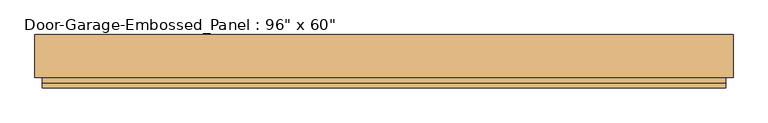
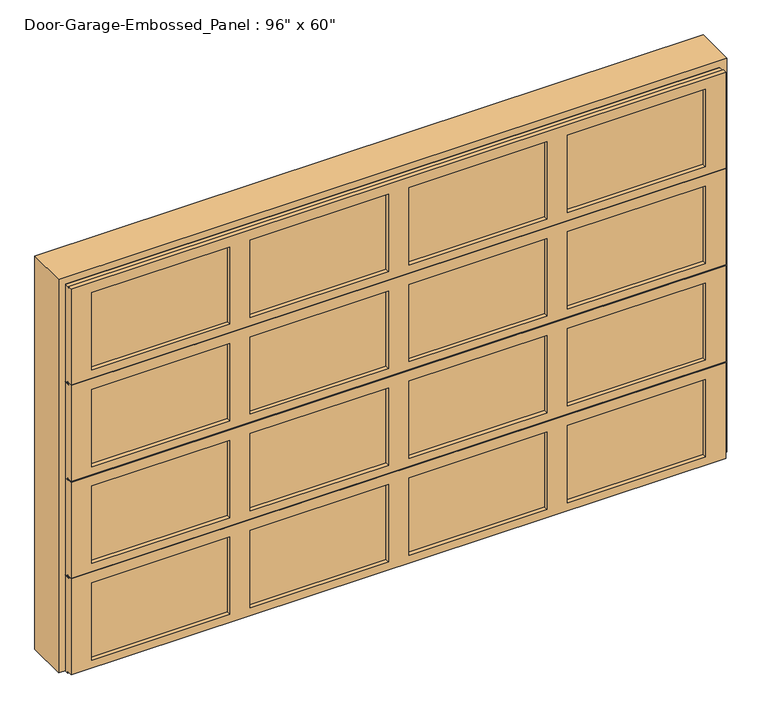
"""IFC4 building model written with IfcOpenShell, lengths in millimetres: door geometry."""

from ifc_helpers import new_model, si_unit, frame, origin, place, context, project, spatial, polyline, outline, extrude, faceted_brep, source, transform, mapped, element, save


def door_11e1ca51(model_context):
    return source(origin(), model_context, "Body", "SolidModel", [
        extrude(outline(polyline([(552.45, -95.25), (552.45, -101.6), (38.1, -101.6), (38.1, -95.25), (552.45, -95.25)])), frame((0.0, 0.0, 1181.1), z_axis=(0.0, 0.0, 1.0), x_axis=(1.0, 0.0, 0.0)), (0.0, 0.0, 1.0), 304.8),
        extrude(outline(polyline([(-38.1, -95.25), (-38.1, -101.6), (-552.45, -101.6), (-552.45, -95.25), (-38.1, -95.25)])), frame((0.0, 0.0, 1181.1), z_axis=(0.0, 0.0, 1.0), x_axis=(1.0, 0.0, 0.0)), (0.0, 0.0, 1.0), 304.8),
        extrude(outline(polyline([(1143.0, -95.25), (1143.0, -101.6), (628.65, -101.6), (628.65, -95.25), (1143.0, -95.25)])), frame((0.0, 0.0, 1181.1), z_axis=(0.0, 0.0, 1.0), x_axis=(1.0, 0.0, 0.0)), (0.0, 0.0, 1.0), 304.8),
        extrude(outline(polyline([(-628.65, -95.25), (-628.65, -101.6), (-1143.0, -101.6), (-1143.0, -95.25), (-628.65, -95.25)])), frame((0.0, 0.0, 1181.1), z_axis=(0.0, 0.0, 1.0), x_axis=(1.0, 0.0, 0.0)), (0.0, 0.0, 1.0), 304.8),
        faceted_brep([(1219.2, -101.6, 1527.175), (1219.2, -117.475, 1527.175), (1219.2, -117.475, 1149.35), (1219.2, -95.25, 1149.35), (1219.2, -95.25, 1143.0), (1219.2, -79.375, 1143.0), (1219.2, -79.375, 1520.825), (1219.2, -101.6, 1520.825), (-1219.2, -117.475, 1527.175), (-1219.2, -101.6, 1527.175), (-1219.2, -101.6, 1520.825), (-1219.2, -79.375, 1520.825), (-1219.2, -79.375, 1143.0), (-1219.2, -95.25, 1143.0), (-1219.2, -95.25, 1149.35), (-1219.2, -117.475, 1149.35), (628.65, -117.475, 1485.9), (1143.0, -117.475, 1485.9), (1143.0, -117.475, 1181.1), (628.65, -117.475, 1181.1), (-552.45, -117.475, 1485.9), (-38.1, -117.475, 1485.9), (-38.1, -117.475, 1181.1), (-552.45, -117.475, 1181.1), (38.1, -117.475, 1485.9), (552.45, -117.475, 1485.9), (552.45, -117.475, 1181.1), (38.1, -117.475, 1181.1), (-1143.0, -117.475, 1485.9), (-628.65, -117.475, 1485.9), (-628.65, -117.475, 1181.1), (-1143.0, -117.475, 1181.1), (1143.0, -79.375, 1485.9), (628.65, -79.375, 1485.9), (628.65, -79.375, 1181.1), (1143.0, -79.375, 1181.1), (-38.1, -79.375, 1485.9), (-552.45, -79.375, 1485.9), (-552.45, -79.375, 1181.1), (-38.1, -79.375, 1181.1), (552.45, -79.375, 1485.9), (38.1, -79.375, 1485.9), (38.1, -79.375, 1181.1), (552.45, -79.375, 1181.1), (-628.65, -79.375, 1485.9), (-1143.0, -79.375, 1485.9), (-1143.0, -79.375, 1181.1), (-628.65, -79.375, 1181.1)], [[[0, 1, 2, 3, 4, 5, 6, 7]], [[8, 9, 10, 11, 12, 13, 14, 15]], [[1, 0, 9, 8]], [[2, 1, 8, 15], [16, 17, 18, 19], [20, 21, 22, 23], [24, 25, 26, 27], [28, 29, 30, 31]], [[3, 2, 15, 14]], [[4, 3, 14, 13]], [[5, 4, 13, 12]], [[6, 5, 12, 11], [32, 33, 34, 35], [36, 37, 38, 39], [40, 41, 42, 43], [44, 45, 46, 47]], [[7, 6, 11, 10]], [[0, 7, 10, 9]], [[16, 33, 32, 17]], [[33, 16, 19, 34]], [[34, 19, 18, 35]], [[17, 32, 35, 18]], [[20, 37, 36, 21]], [[37, 20, 23, 38]], [[38, 23, 22, 39]], [[21, 36, 39, 22]], [[24, 41, 40, 25]], [[41, 24, 27, 42]], [[42, 27, 26, 43]], [[25, 40, 43, 26]], [[28, 45, 44, 29]], [[45, 28, 31, 46]], [[46, 31, 30, 47]], [[29, 44, 47, 30]]]),
        extrude(outline(polyline([(552.45, -95.25), (552.45, -101.6), (38.1, -101.6), (38.1, -95.25), (552.45, -95.25)])), frame((0.0, 0.0, 800.1), z_axis=(0.0, 0.0, 1.0), x_axis=(1.0, 0.0, 0.0)), (0.0, 0.0, 1.0), 304.8),
        extrude(outline(polyline([(-38.1, -95.25), (-38.1, -101.6), (-552.45, -101.6), (-552.45, -95.25), (-38.1, -95.25)])), frame((0.0, 0.0, 800.1), z_axis=(0.0, 0.0, 1.0), x_axis=(1.0, 0.0, 0.0)), (0.0, 0.0, 1.0), 304.8),
        extrude(outline(polyline([(1143.0, -95.25), (1143.0, -101.6), (628.65, -101.6), (628.65, -95.25), (1143.0, -95.25)])), frame((0.0, 0.0, 800.1), z_axis=(0.0, 0.0, 1.0), x_axis=(1.0, 0.0, 0.0)), (0.0, 0.0, 1.0), 304.8),
        extrude(outline(polyline([(-628.65, -95.25), (-628.65, -101.6), (-1143.0, -101.6), (-1143.0, -95.25), (-628.65, -95.25)])), frame((0.0, 0.0, 800.1), z_axis=(0.0, 0.0, 1.0), x_axis=(1.0, 0.0, 0.0)), (0.0, 0.0, 1.0), 304.8),
        faceted_brep([(1219.2, -101.6, 1146.175), (1219.2, -117.475, 1146.175), (1219.2, -117.475, 768.35), (1219.2, -95.25, 768.35), (1219.2, -95.25, 762.0), (1219.2, -79.375, 762.0), (1219.2, -79.375, 1139.825), (1219.2, -101.6, 1139.825), (-1219.2, -117.475, 1146.175), (-1219.2, -101.6, 1146.175), (-1219.2, -101.6, 1139.825), (-1219.2, -79.375, 1139.825), (-1219.2, -79.375, 762.0), (-1219.2, -95.25, 762.0), (-1219.2, -95.25, 768.35), (-1219.2, -117.475, 768.35), (628.65, -117.475, 1104.9), (1143.0, -117.475, 1104.9), (1143.0, -117.475, 800.1), (628.65, -117.475, 800.1), (-552.45, -117.475, 1104.9), (-38.1, -117.475, 1104.9), (-38.1, -117.475, 800.1), (-552.45, -117.475, 800.1), (38.1, -117.475, 1104.9), (552.45, -117.475, 1104.9), (552.45, -117.475, 800.1), (38.1, -117.475, 800.1), (-1143.0, -117.475, 1104.9), (-628.65, -117.475, 1104.9), (-628.65, -117.475, 800.1), (-1143.0, -117.475, 800.1), (1143.0, -79.375, 1104.9), (628.65, -79.375, 1104.9), (628.65, -79.375, 800.1), (1143.0, -79.375, 800.1), (-38.1, -79.375, 1104.9), (-552.45, -79.375, 1104.9), (-552.45, -79.375, 800.1), (-38.1, -79.375, 800.1), (552.45, -79.375, 1104.9), (38.1, -79.375, 1104.9), (38.1, -79.375, 800.1), (552.45, -79.375, 800.1), (-628.65, -79.375, 1104.9), (-1143.0, -79.375, 1104.9), (-1143.0, -79.375, 800.1), (-628.65, -79.375, 800.1)], [[[0, 1, 2, 3, 4, 5, 6, 7]], [[8, 9, 10, 11, 12, 13, 14, 15]], [[1, 0, 9, 8]], [[2, 1, 8, 15], [16, 17, 18, 19], [20, 21, 22, 23], [24, 25, 26, 27], [28, 29, 30, 31]], [[3, 2, 15, 14]], [[4, 3, 14, 13]], [[5, 4, 13, 12]], [[6, 5, 12, 11], [32, 33, 34, 35], [36, 37, 38, 39], [40, 41, 42, 43], [44, 45, 46, 47]], [[7, 6, 11, 10]], [[0, 7, 10, 9]], [[16, 33, 32, 17]], [[33, 16, 19, 34]], [[34, 19, 18, 35]], [[17, 32, 35, 18]], [[20, 37, 36, 21]], [[37, 20, 23, 38]], [[38, 23, 22, 39]], [[21, 36, 39, 22]], [[24, 41, 40, 25]], [[41, 24, 27, 42]], [[42, 27, 26, 43]], [[25, 40, 43, 26]], [[28, 45, 44, 29]], [[45, 28, 31, 46]], [[46, 31, 30, 47]], [[29, 44, 47, 30]]]),
        extrude(outline(polyline([(552.45, -95.25), (552.45, -101.6), (38.1, -101.6), (38.1, -95.25), (552.45, -95.25)])), frame((0.0, 0.0, 419.1), z_axis=(0.0, 0.0, 1.0), x_axis=(1.0, 0.0, 0.0)), (0.0, 0.0, 1.0), 304.8),
        extrude(outline(polyline([(-38.1, -95.25), (-38.1, -101.6), (-552.45, -101.6), (-552.45, -95.25), (-38.1, -95.25)])), frame((0.0, 0.0, 419.1), z_axis=(0.0, 0.0, 1.0), x_axis=(1.0, 0.0, 0.0)), (0.0, 0.0, 1.0), 304.8),
        extrude(outline(polyline([(1143.0, -95.25), (1143.0, -101.6), (628.65, -101.6), (628.65, -95.25), (1143.0, -95.25)])), frame((0.0, 0.0, 419.1), z_axis=(0.0, 0.0, 1.0), x_axis=(1.0, 0.0, 0.0)), (0.0, 0.0, 1.0), 304.8),
        extrude(outline(polyline([(-628.65, -95.25), (-628.65, -101.6), (-1143.0, -101.6), (-1143.0, -95.25), (-628.65, -95.25)])), frame((0.0, 0.0, 419.1), z_axis=(0.0, 0.0, 1.0), x_axis=(1.0, 0.0, 0.0)), (0.0, 0.0, 1.0), 304.8),
        faceted_brep([(1219.2, -101.6, 765.175), (1219.2, -117.475, 765.175), (1219.2, -117.475, 387.35), (1219.2, -95.25, 387.35), (1219.2, -95.25, 381.0), (1219.2, -79.375, 381.0), (1219.2, -79.375, 758.825), (1219.2, -101.6, 758.825), (-1219.2, -117.475, 765.175), (-1219.2, -101.6, 765.175), (-1219.2, -101.6, 758.825), (-1219.2, -79.375, 758.825), (-1219.2, -79.375, 381.0), (-1219.2, -95.25, 381.0), (-1219.2, -95.25, 387.35), (-1219.2, -117.475, 387.35), (628.65, -117.475, 723.9), (1143.0, -117.475, 723.9), (1143.0, -117.475, 419.1), (628.65, -117.475, 419.1), (-552.45, -117.475, 723.9), (-38.1, -117.475, 723.9), (-38.1, -117.475, 419.1), (-552.45, -117.475, 419.1), (38.1, -117.475, 723.9), (552.45, -117.475, 723.9), (552.45, -117.475, 419.1), (38.1, -117.475, 419.1), (-1143.0, -117.475, 723.9), (-628.65, -117.475, 723.9), (-628.65, -117.475, 419.1), (-1143.0, -117.475, 419.1), (1143.0, -79.375, 723.9), (628.65, -79.375, 723.9), (628.65, -79.375, 419.1), (1143.0, -79.375, 419.1), (-38.1, -79.375, 723.9), (-552.45, -79.375, 723.9), (-552.45, -79.375, 419.1), (-38.1, -79.375, 419.1), (552.45, -79.375, 723.9), (38.1, -79.375, 723.9), (38.1, -79.375, 419.1), (552.45, -79.375, 419.1), (-628.65, -79.375, 723.9), (-1143.0, -79.375, 723.9), (-1143.0, -79.375, 419.1), (-628.65, -79.375, 419.1)], [[[0, 1, 2, 3, 4, 5, 6, 7]], [[8, 9, 10, 11, 12, 13, 14, 15]], [[1, 0, 9, 8]], [[2, 1, 8, 15], [16, 17, 18, 19], [20, 21, 22, 23], [24, 25, 26, 27], [28, 29, 30, 31]], [[3, 2, 15, 14]], [[4, 3, 14, 13]], [[5, 4, 13, 12]], [[6, 5, 12, 11], [32, 33, 34, 35], [36, 37, 38, 39], [40, 41, 42, 43], [44, 45, 46, 47]], [[7, 6, 11, 10]], [[0, 7, 10, 9]], [[16, 33, 32, 17]], [[33, 16, 19, 34]], [[34, 19, 18, 35]], [[17, 32, 35, 18]], [[20, 37, 36, 21]], [[37, 20, 23, 38]], [[38, 23, 22, 39]], [[21, 36, 39, 22]], [[24, 41, 40, 25]], [[41, 24, 27, 42]], [[42, 27, 26, 43]], [[25, 40, 43, 26]], [[28, 45, 44, 29]], [[45, 28, 31, 46]], [[46, 31, 30, 47]], [[29, 44, 47, 30]]]),
        extrude(outline(polyline([(552.45, -95.25), (552.45, -101.6), (38.1, -101.6), (38.1, -95.25), (552.45, -95.25)])), frame((0.0, 0.0, 38.1), z_axis=(0.0, 0.0, 1.0), x_axis=(1.0, 0.0, 0.0)), (0.0, 0.0, 1.0), 304.8),
        extrude(outline(polyline([(-38.1, -95.25), (-38.1, -101.6), (-552.45, -101.6), (-552.45, -95.25), (-38.1, -95.25)])), frame((0.0, 0.0, 38.1), z_axis=(0.0, 0.0, 1.0), x_axis=(1.0, 0.0, 0.0)), (0.0, 0.0, 1.0), 304.8),
        extrude(outline(polyline([(1143.0, -95.25), (1143.0, -101.6), (628.65, -101.6), (628.65, -95.25), (1143.0, -95.25)])), frame((0.0, 0.0, 38.1), z_axis=(0.0, 0.0, 1.0), x_axis=(1.0, 0.0, 0.0)), (0.0, 0.0, 1.0), 304.8),
        extrude(outline(polyline([(-628.65, -95.25), (-628.65, -101.6), (-1143.0, -101.6), (-1143.0, -95.25), (-628.65, -95.25)])), frame((0.0, 0.0, 38.1), z_axis=(0.0, 0.0, 1.0), x_axis=(1.0, 0.0, 0.0)), (0.0, 0.0, 1.0), 304.8),
        faceted_brep([(1219.2, -101.6, 384.175), (1219.2, -117.475, 384.175), (1219.2, -117.475, 6.35), (1219.2, -95.25, 6.35), (1219.2, -95.25, 0.0), (1219.2, -79.375, 0.0), (1219.2, -79.375, 377.825), (1219.2, -101.6, 377.825), (-1219.2, -117.475, 384.175), (-1219.2, -101.6, 384.175), (-1219.2, -101.6, 377.825), (-1219.2, -79.375, 377.825), (-1219.2, -79.375, 0.0), (-1219.2, -95.25, 0.0), (-1219.2, -95.25, 6.35), (-1219.2, -117.475, 6.35), (628.65, -117.475, 342.9), (1143.0, -117.475, 342.9), (1143.0, -117.475, 38.1), (628.65, -117.475, 38.1), (-552.45, -117.475, 342.9), (-38.1, -117.475, 342.9), (-38.1, -117.475, 38.1), (-552.45, -117.475, 38.1), (38.1, -117.475, 342.9), (552.45, -117.475, 342.9), (552.45, -117.475, 38.1), (38.1, -117.475, 38.1), (-1143.0, -117.475, 342.9), (-628.65, -117.475, 342.9), (-628.65, -117.475, 38.1), (-1143.0, -117.475, 38.1), (1143.0, -79.375, 342.9), (628.65, -79.375, 342.9), (628.65, -79.375, 38.1), (1143.0, -79.375, 38.1), (-38.1, -79.375, 342.9), (-552.45, -79.375, 342.9), (-552.45, -79.375, 38.1), (-38.1, -79.375, 38.1), (552.45, -79.375, 342.9), (38.1, -79.375, 342.9), (38.1, -79.375, 38.1), (552.45, -79.375, 38.1), (-628.65, -79.375, 342.9), (-1143.0, -79.375, 342.9), (-1143.0, -79.375, 38.1), (-628.65, -79.375, 38.1)], [[[0, 1, 2, 3, 4, 5, 6, 7]], [[8, 9, 10, 11, 12, 13, 14, 15]], [[1, 0, 9, 8]], [[2, 1, 8, 15], [16, 17, 18, 19], [20, 21, 22, 23], [24, 25, 26, 27], [28, 29, 30, 31]], [[3, 2, 15, 14]], [[4, 3, 14, 13]], [[5, 4, 13, 12]], [[6, 5, 12, 11], [32, 33, 34, 35], [36, 37, 38, 39], [40, 41, 42, 43], [44, 45, 46, 47]], [[7, 6, 11, 10]], [[0, 7, 10, 9]], [[16, 33, 32, 17]], [[33, 16, 19, 34]], [[34, 19, 18, 35]], [[17, 32, 35, 18]], [[20, 37, 36, 21]], [[37, 20, 23, 38]], [[38, 23, 22, 39]], [[21, 36, 39, 22]], [[24, 41, 40, 25]], [[41, 24, 27, 42]], [[42, 27, 26, 43]], [[25, 40, 43, 26]], [[28, 45, 44, 29]], [[45, 28, 31, 46]], [[46, 31, 30, 47]], [[29, 44, 47, 30]]]),
        extrude(outline(polyline([(0.0, 1219.2), (0.0, 1244.6), (1549.4, 1244.6), (1549.4, -1244.6), (0.0, -1244.6), (0.0, -1219.2), (1524.0, -1219.2), (1524.0, 1219.2), (0.0, 1219.2)])), frame((0.0, -79.375, 0.0), z_axis=(0.0, 1.0, 0.0), x_axis=(0.0, 0.0, 1.0)), (0.0, 0.0, 1.0), 152.4),
    ])


if __name__ == "__main__":
    model = new_model("IFC4")
    model_context = context("Model", 3, world=origin())
    ifc_project = project(units=[si_unit("LENGTHUNIT", "METRE", prefix="MILLI")], contexts=[model_context])
    site = spatial("IfcSite", under=ifc_project)
    building = spatial("IfcBuilding", under=site)
    placement = place(None, origin())
    door_shape = door_11e1ca51(model_context)
    element("IfcDoor", 1, ObjectType="Door-Garage-Embossed_Panel : 96\" x 60\"", at=placement, inside=building, context=model_context, shape_type="MappedRepresentation", body=[
        mapped(door_shape, transform((0.0, 0.0, 0.0), x_axis=(1.0, 0.0, 0.0), y_axis=(0.0, 1.0, 0.0), z_axis=(0.0, 0.0, 1.0))),
    ])
    save(model, "model.ifc")

# Revit data of these elements
# Type "Door-Garage-Embossed_Panel : 96\" x 60\""
#   Type Mark = "10"
#   Assembly Code = "B2030400"
#   Analytic Construction = "Metal"
#   Thickness = 0' - 1 1/2"
#   Thermal Resistance (R) = 1.5338 (h·ft²·°F)/BTU
#   Rough Width = 8' - 2"
#   Rough Height = 5' - 1"
#   Panel Height = 1' - 3"
#   Height = 5' - 0"
#   Width = 8' - 0"
#   Heat Transfer Coefficient (U) = 0.6520 BTU/(h·ft²·°F)
#   Panels = 4
#   Function = 1
#   Exterior Trim [instance default] = yes
#   Trim Material = Steel, Paint Finish, Ivory, Matte
#   Panel Material = Steel, Paint Finish, Ivory, Matte
#   Frame Material = Steel, Paint Finish, Ivory, Matte
#   Visual Light Transmittance = 0
#   Solar Heat Gain Coefficient = 0
#   Wall Closure = (empty or 0)
# Element 1 (IfcDoor, "Door-Garage-Embossed_Panel : 96\" x 60\"")
#   Materials on its faces: "Steel, Paint Finish, Ivory, Matte"
# Materials
#   "Steel, Paint Finish, Ivory, Matte": class "Metal", colour RGB 247 247 239, transparency 0, Description = "Steel, paint finish, ivory, matte", Cost = 0
